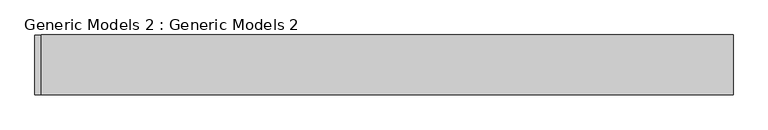
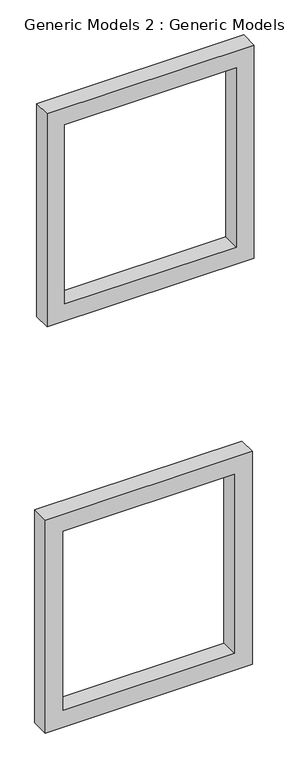
"""IFC4 building model written with IfcOpenShell, lengths in millimetres: proxy geometry, Generic Models 2 : Generic Models 2."""

from ifc_helpers import new_model, si_unit, frame, origin, place, context, project, spatial, polyline, outline, extrude, source, transform, mapped, element, save


def generic_models_2_generic_models_2_8f6bc761(model_context):
    return source(origin(), model_context, "Body", "SweptSolid", [
        extrude(outline(polyline([(5740.4, -7437.0719939), (5740.4, -8910.2719939), (4140.2, -8910.2719939), (4140.2, -7437.0719939), (5740.4, -7437.0719939)]), holes=[polyline([(5613.4, -7564.0719939), (4267.2, -7564.0719939), (4267.2, -8783.2719939), (5613.4, -8783.2719939), (5613.4, -7564.0719939)])]), frame((0.0, -5849.5827462, 0.0), z_axis=(0.0, 1.0, 0.0), x_axis=(0.0, 0.0, 1.0)), (0.0, 0.0, 1.0), 127.0),
        extrude(outline(polyline([(2692.4, -7450.2482439), (2692.4, -8923.4482439), (1092.2, -8923.4482439), (1092.2, -7450.2482439), (2692.4, -7450.2482439)]), holes=[polyline([(2565.4, -7577.2482439), (1219.2, -7577.2482439), (1219.2, -8796.4482439), (2565.4, -8796.4482439), (2565.4, -7577.2482439)])]), frame((0.0, -5849.5827462, 0.0), z_axis=(0.0, 1.0, 0.0), x_axis=(0.0, 0.0, 1.0)), (0.0, 0.0, 1.0), 127.0),
    ])


if __name__ == "__main__":
    model = new_model("IFC4")
    model_context = context("Model", 3, world=origin())
    ifc_project = project(units=[si_unit("LENGTHUNIT", "METRE", prefix="MILLI")], contexts=[model_context])
    site = spatial("IfcSite", under=ifc_project)
    building = spatial("IfcBuilding", under=site)
    placement = place(None, origin())
    generic_models_2_generic_models_2_shape = generic_models_2_generic_models_2_8f6bc761(model_context)
    element("IfcBuildingElementProxy", 1, Name="Generic Models 2 : Generic Models 2", ObjectType="Generic Models 2 : Generic Models 2", at=placement, inside=building, context=model_context, shape_type="MappedRepresentation", body=[
        mapped(generic_models_2_generic_models_2_shape, transform((0.0, 0.0, 0.0), x_axis=(1.0, 0.0, 0.0), y_axis=(0.0, 1.0, 0.0), z_axis=(0.0, 0.0, 1.0))),
    ])
    save(model, "model.ifc")

# Revit data of these elements
# Element 1 (IfcBuildingElementProxy, "Generic Models 2 : Generic Models 2")
#   Materials on its faces: "BLACK"
# Materials
#   "BLACK": class "Generic", colour RGB 120 120 120, transparency 0, Cost = 0
